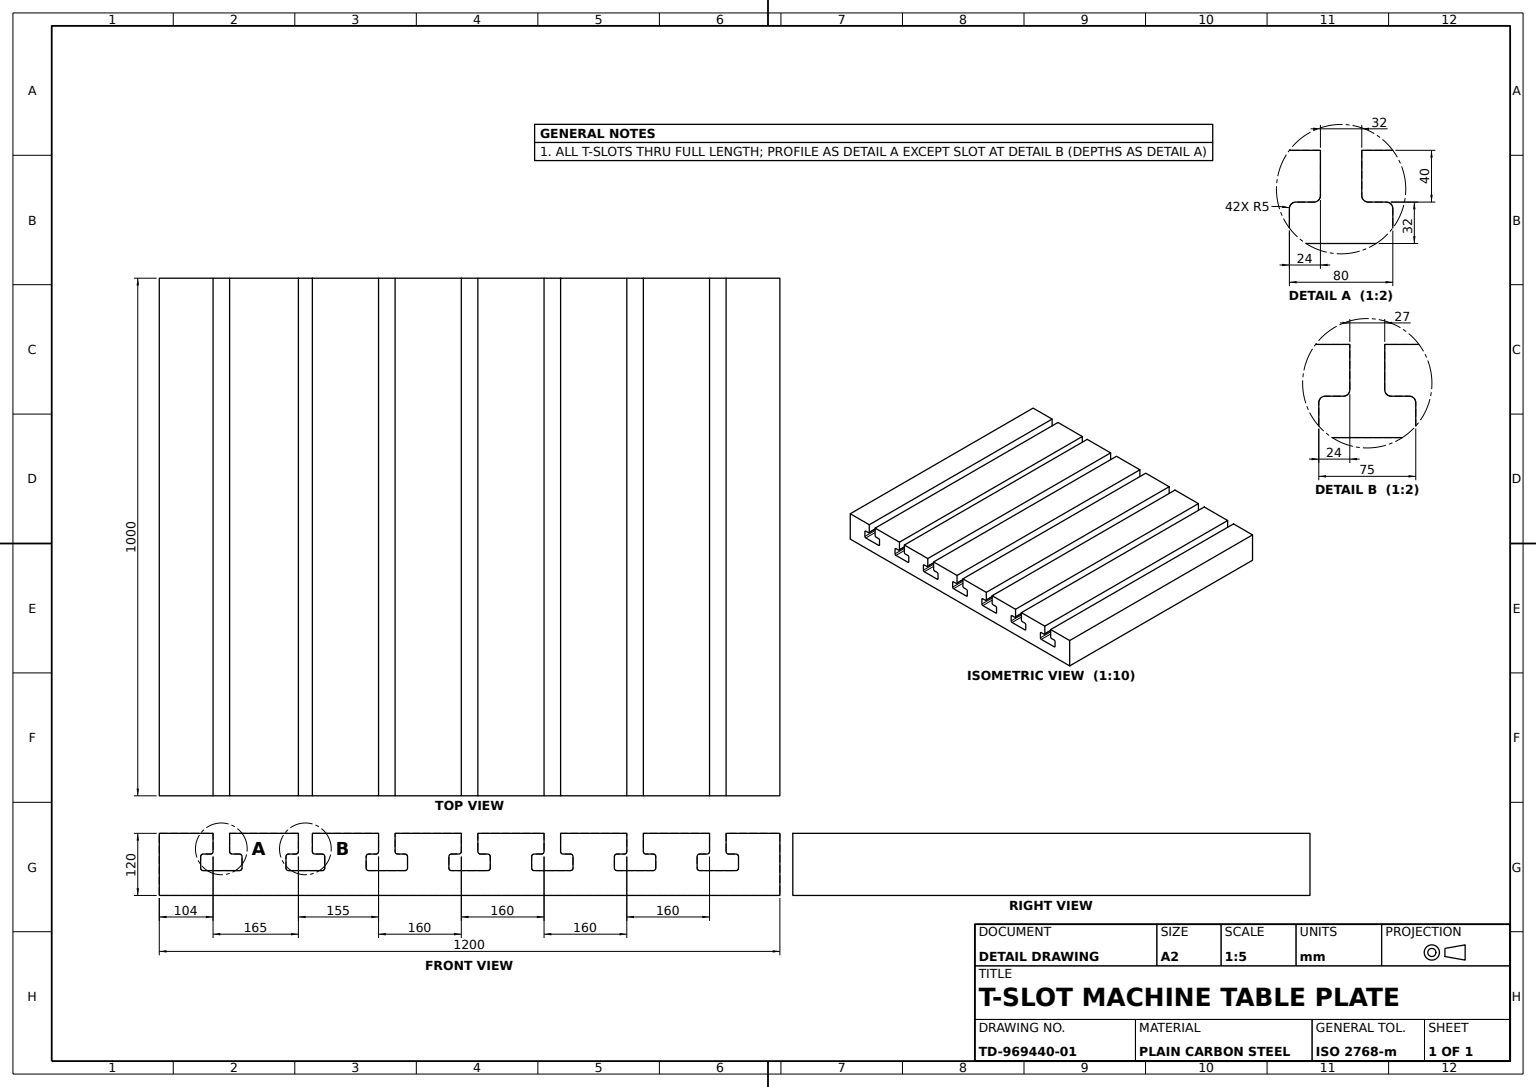
SolidWorks part; units mm, degrees
material "Plain Carbon Steel"
ref_plane "Front Plane" through (0, 0, 0) normal (0, 0, 1) x (1, 0, 0)
ref_plane "Top Plane" through (0, 0, 0) normal (0, 1, 0) x (1, 0, 0)
ref_plane "Right Plane" through (0, 0, 0) normal (1, 0, 0) x (0, 0, -1)
sketch "Plate Outline Sketch" plane through (0, 0, 0) normal (0, 0, 1) x (1, 0, 0)
  line L0 (0, 0) -> (1200, 0)
  line L1 (1200, 0) -> (1200, 1000)
  line L2 (1200, 1000) -> (0, 1000)
  line L3 (0, 1000) -> (0, 0)
  dimension "D1" = 1200
  dimension "D2" = 1000
  dimension "D3" = 1200
extrude "Base Plate 120mm" add sketch "Plate Outline Sketch" along normal blind 120
sketch "T-Slot Profiles Set A Sketch" plane through (0, 0, 0) normal (0, -1, 0) x (1, 0, 0)
  line L0 (0, 0) -> (120, 0)
  line L1 (0, 0) -> (1200, 0) construction
  line L3 (0, 120) -> (1200, 120) construction
  line L5 (85, 80) -> (99, 80)
  line L8 (136, 120) -> (136, 85)
  line L10 (160, 53) -> (160, 75)
  line L11 (80, 75) -> (80, 53)
  line L13 (104, 120) -> (104, 85)
  line L14 (141, 80) -> (155, 80)
  line L15 (104, 120) -> (136, 120)
  line L16 (85, 48) -> (155, 48)
  line L17 (0, 120) -> (104, 120)
  arc A0 (155, 48) -> (160, 53) centre (155, 53) ccw
  arc A1 (85, 48) -> (80, 53) centre (85, 53) cw
  arc A2 (160, 75) -> (155, 80) centre (155, 75) ccw
  arc A3 (141, 80) -> (136, 85) centre (141, 85) cw
  arc A4 (99, 80) -> (104, 85) centre (99, 85) ccw
  arc A5 (85, 80) -> (80, 75) centre (85, 75) ccw
  point P12 (120, 80)
  point P24 (136, 80)
  line M9 (1200, 120) -> (0, 120)
  dimension "D2" = 5
  dimension "D7" = 5
  dimension "D1" = 120
  dimension "D3" = 32
  dimension "D4" = 40
  dimension "D5" = 24
  dimension "D6" = 32
  dimension "D8" = 16
  dimension "D9" = 80
extrude "T-Slots Set A" cut sketch "T-Slot Profiles Set A Sketch" against normal blind 1000 contours L5 A5 L11 A1 L16 A0 L10 A2 L14 A3 L8 L13 A4 M9
sketch "T-Slot Profiles Set B Sketch" plane through (0, 0, 0) normal (0, -1, 0) x (1, 0, 0)
  line L0 (0, 120) -> (0, 0) construction
  line L1 (0, 0) -> (1200, 0) construction
  line L3 (136, 120) -> (1200, 120) construction
  line L4 (269, 120) -> (296, 120)
  line L5 (296, 120) -> (296, 85)
  line L6 (250, 48) -> (280, 48)
  line L7 (320, 53) -> (320, 75)
  line L8 (315, 80) -> (301, 80)
  line L9 (245, 53) -> (245, 75)
  line L10 (250, 80) -> (264, 80)
  line L11 (269, 85) -> (269, 120)
  line L12 (280, 48) -> (315, 48)
  line L14 (424, 120) -> (456, 120)
  line L15 (456, 120) -> (456, 85)
  line L16 (424, 120) -> (424, 85)
  line L18 (480, 53) -> (480, 75)
  line L19 (475, 80) -> (461, 80)
  line L20 (400, 53) -> (400, 75)
  line L21 (405, 80) -> (419, 80)
  line L22 (440, 48) -> (475, 48)
  line L24 (584, 120) -> (616, 120)
  line L25 (616, 120) -> (616, 85)
  line L26 (584, 120) -> (584, 85)
  line L28 (640, 53) -> (640, 75)
  line L29 (635, 80) -> (621, 80)
  line L30 (560, 53) -> (560, 75)
  line L31 (565, 80) -> (579, 80)
  line L32 (600, 48) -> (635, 48)
  line L34 (744, 120) -> (776, 120)
  line L35 (776, 120) -> (776, 85)
  line L36 (744, 120) -> (744, 85)
  line L38 (800, 53) -> (800, 75)
  line L39 (795, 80) -> (781, 80)
  line L40 (720, 53) -> (720, 75)
  line L41 (725, 80) -> (739, 80)
  line L42 (760, 48) -> (795, 48)
  line L44 (904, 120) -> (936, 120)
  line L45 (936, 120) -> (936, 85)
  line L47 (960, 53) -> (960, 75)
  line L48 (955, 80) -> (941, 80)
  line L49 (880, 53) -> (880, 75)
  line L50 (885, 80) -> (899, 80)
  line L51 (904, 85) -> (904, 120)
  line L52 (920, 48) -> (955, 48)
  line L54 (1064, 120) -> (1096, 120)
  line L55 (1096, 120) -> (1096, 85)
  line L56 (1080, 48) -> (1115, 48)
  line L57 (1120, 53) -> (1120, 75)
  line L58 (1115, 80) -> (1101, 80)
  line L59 (1040, 53) -> (1040, 75)
  line L60 (1045, 80) -> (1059, 80)
  line L61 (1064, 85) -> (1064, 120)
  line L62 (405, 48) -> (440, 48)
  line L63 (565, 48) -> (600, 48)
  line L64 (725, 48) -> (760, 48)
  line L65 (885, 48) -> (920, 48)
  line L66 (1045, 48) -> (1080, 48)
  arc A0 (301, 80) -> (296, 85) centre (301, 85) cw
  arc A1 (264, 80) -> (269, 85) centre (264, 85) ccw
  arc A2 (315, 48) -> (320, 53) centre (315, 53) ccw
  arc A3 (320, 75) -> (315, 80) centre (315, 75) ccw
  arc A4 (250, 48) -> (245, 53) centre (250, 53) cw
  arc A5 (250, 80) -> (245, 75) centre (250, 75) ccw
  arc A6 (899, 80) -> (904, 85) centre (899, 85) ccw
  arc A7 (941, 80) -> (936, 85) centre (941, 85) cw
  arc A8 (960, 75) -> (955, 80) centre (955, 75) ccw
  arc A9 (955, 48) -> (960, 53) centre (955, 53) ccw
  arc A10 (885, 48) -> (880, 53) centre (885, 53) cw
  arc A11 (885, 80) -> (880, 75) centre (885, 75) ccw
  arc A12 (1045, 80) -> (1040, 75) centre (1045, 75) ccw
  arc A13 (1045, 48) -> (1040, 53) centre (1045, 53) cw
  arc A14 (1115, 48) -> (1120, 53) centre (1115, 53) ccw
  arc A15 (1120, 75) -> (1115, 80) centre (1115, 75) ccw
  arc A16 (1101, 80) -> (1096, 85) centre (1101, 85) cw
  arc A17 (1059, 80) -> (1064, 85) centre (1059, 85) ccw
  arc A18 (725, 48) -> (720, 53) centre (725, 53) cw
  arc A19 (720, 75) -> (725, 80) centre (725, 75) cw
  arc A20 (739, 80) -> (744, 85) centre (739, 85) ccw
  arc A21 (795, 48) -> (800, 53) centre (795, 53) ccw
  arc A22 (800, 75) -> (795, 80) centre (795, 75) ccw
  arc A23 (781, 80) -> (776, 85) centre (781, 85) cw
  arc A24 (579, 80) -> (584, 85) centre (579, 85) ccw
  arc A25 (621, 80) -> (616, 85) centre (621, 85) cw
  arc A26 (640, 75) -> (635, 80) centre (635, 75) ccw
  arc A27 (635, 48) -> (640, 53) centre (635, 53) ccw
  arc A28 (565, 48) -> (560, 53) centre (565, 53) cw
  arc A29 (560, 75) -> (565, 80) centre (565, 75) cw
  arc A30 (405, 48) -> (400, 53) centre (405, 53) cw
  arc A31 (405, 80) -> (400, 75) centre (405, 75) ccw
  arc A32 (475, 48) -> (480, 53) centre (475, 53) ccw
  arc A33 (480, 75) -> (475, 80) centre (475, 75) ccw
  arc A34 (461, 80) -> (456, 85) centre (461, 85) cw
  arc A35 (419, 80) -> (424, 85) centre (419, 85) ccw
  point P3 (296, 80)
  point P10 (282.5, 120)
  point P14 (280, 48)
  point P22 (440, 120)
  point P27 (440, 48)
  point P34 (600, 120)
  point P39 (600, 48)
  point P46 (760, 120)
  point P51 (760, 48)
  point P58 (920, 120)
  point P62 (920, 48)
  point P70 (1080, 120)
  point P73 (1080, 48)
  point P89 (960, 48)
  point P100 (1120, 48)
  point P115 (800, 48)
  point P128 (640, 48)
  point P139 (480, 48)
  dimension "D2" = 5
  dimension "D4" = 5
  dimension "D6" = 5
  dimension "D9" = 5
  dimension "D12" = 5
  dimension "D15" = 5
  dimension "D18" = 5
  dimension "D27" = 320
  dimension "D30" = 65
  dimension "D3" = 40
  dimension "D5" = 160
  dimension "D7" = 40
  dimension "D8" = 160
  dimension "D10" = 40
  dimension "D11" = 160
  dimension "D13" = 40
  dimension "D14" = 160
  dimension "D16" = 40
  dimension "D17" = 160
  dimension "D19" = 40
  dimension "D20" = 27
  dimension "D21" = 72
  dimension "D22" = 75
  dimension "D23" = 24
  dimension "D24" = 104
  dimension "D25" = 24
  dimension "D26" = 24
  dimension "D28" = 80
  dimension "D29" = 35
  dimension "D31" = 45
  dimension "D32" = 37
  dimension "D33" = 35
  dimension "D34" = 35
  dimension "D35" = 22
  dimension "D36" = 37
  dimension "D37" = 160
  dimension "D38" = 160
  dimension "D39" = 160
  dimension "D40" = 19
  dimension "D41" = 24
  dimension "D42" = 40
  dimension "D43" = 40
  dimension "D44" = 56
  dimension "D45" = 80
  dimension "D46" = 32
  dimension "D47" = 40
  dimension "D48" = 24
  dimension "D49" = 128
  dimension "D50" = 40
  dimension "D51" = 24
  dimension "D52" = 24
  dimension "D53" = 32
  dimension "D54" = 32
  dimension "D55" = 32
extrude "T-Slots Set B" cut sketch "T-Slot Profiles Set B Sketch" against normal blind 1000
